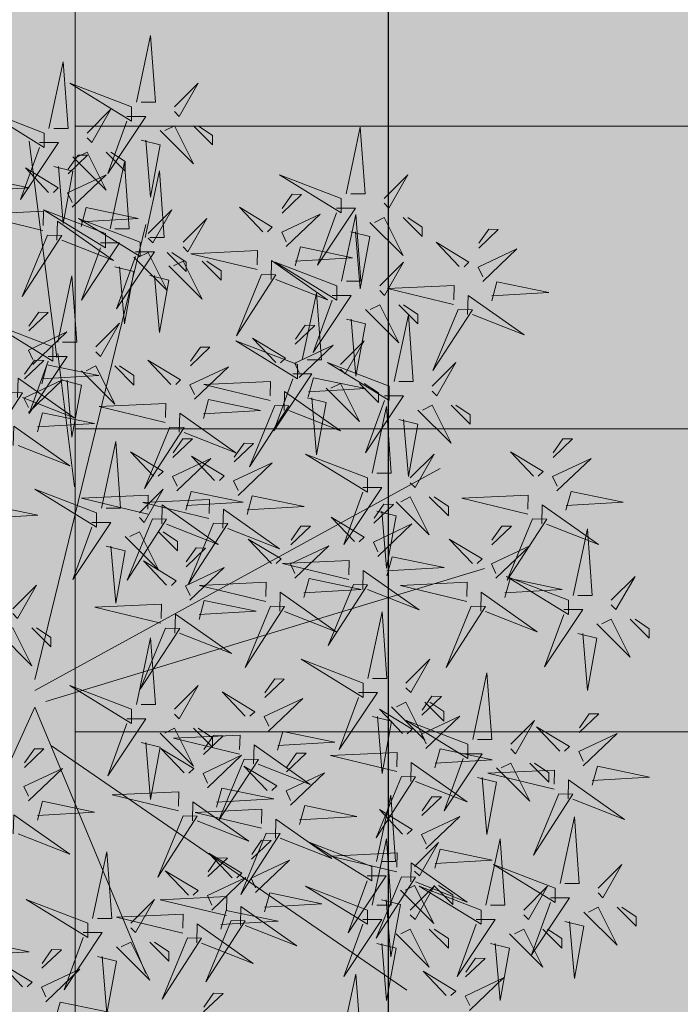
# Model space of a CAD drawing. Units: inches. Extents: x 1704 to 6393, y -157 to 1172.
# Tile 82 of 122: x 2064 to 2081, y 1006 to 1030. Entities that reach past the tile are written whole.
import ezdxf

# ---------------------------------------------------------------- set-up
doc = ezdxf.new("R2010")
doc.units = ezdxf.units.IN
doc.header["$MEASUREMENT"] = 0
for name, color, linetype, lineweight in [('A-ANNO-DIMS', 7, 'Continuous', 13), ('L-DECK-PLNK-PATT', 250, 'Continuous', 13), ('L-HRDS', 8, 'Continuous', 18), ('L-shrub', 74, 'Continuous', 18)]:
    doc.layers.add(name, color=color, linetype=linetype, lineweight=lineweight)
doc.layers.add('L-DECK-PATT', color=35, linetype='Continuous', lineweight=13, true_color=0xa6725b)
doc.layers.add('L-HRDS-PATT', color=9, linetype='Continuous', lineweight=13, true_color=0xc5c1ba)
doc.styles.get("Standard").update_dxf_attribs({"font": 'arial.ttf'})
doc.dimstyles.get("Standard").update_dxf_attribs({"dimtxt": 6, "dimasz": 2, "dimexe": 0.18, "dimexo": 0.0625, "dimgap": 0.09, "dimtad": 0, "dimtih": 1, "dimtoh": 1, "dimdec": 1, "dimzin": 0, "dimdsep": 46, "dimlunit": 3, "dimtxsty": 'Standard', "dimblk": 'ARCHTICK', "dimcen": 0.09, "dimadec": 0, "dimazin": 0, "dimtfac": 1, "dimtdec": 1, "dimtofl": 0, "dimtmove": 0, "dimatfit": 3, "dimfxl": 1, "dimtolj": 1, "dimtzin": 0, "dimarcsym": 0})

# ---------------------------------------------------------------- blocks, each defined once
blk = doc.blocks.new('shrub3')
for p, q in [((-5.99, -2.5), (58.67, 140.12)), ((-14.08, 16.34), (-186.51, 134.74)), ((-5.99, -2.5), (-59.88, 126.66)), ((-11.38, -5.19), (-224.23, -69.78)), ((-5.99, -10.57), (-202.68, -118.21)), ((-5.99, -15.96), (-59.88, -236.62)), ((-17.27, -174.02), (-25.36, -109.43)), ((-16.77, -172.03), (-3.3, -276.98))]:
    blk.add_line(p, q)
for points in [[(-154.93, 159.27), (-161.86, 126.99), (-164.17, 159.27), (-157.24, 159.27)], [(-15.75, 149.73), (-18.28, 140.55), (-43.52, 145.8), (-15.81, 147.42)], [(-217.01, 144.61), (-233.55, 128.86), (-214.88, 137.63), (-217.07, 142.31)], [(-87.91, 145.34), (-97.36, 136.34), (-92.75, 136.22), (-87.97, 143.03)], [(-36.4, 118.43), (-45.64, 120.73), (-41.02, 146.1), (-38.71, 118.43)], [(-227.2, 112.08), (-236.44, 114.38), (-231.82, 139.75), (-229.51, 112.08)], [(-172.08, 112.08), (-181.32, 114.38), (-176.7, 139.75), (-174.39, 112.08)], [(-80.06, 109.47), (-67.78, 139.19), (-86.97, 109.65), (-80.06, 109.47)], [(-11.37, 140.38), (-27.91, 124.63), (-9.24, 133.4), (-11.43, 138.07)], [(-205.66, 137.4), (-194.42, 125.57), (-210.33, 135.21), (-207.96, 137.46)], [(-29.48, 106.9), (-38.71, 106.9), (-20.24, 134.57), (-29.48, 109.2)], [(-263.24, 101.49), (-272.48, 103.79), (-267.86, 129.16), (-265.55, 101.49)], [(-101.26, 101), (-88.98, 130.72), (-108.17, 101.18), (-101.26, 101)], [(-45.64, 113.82), (-61.8, 129.96), (-52.56, 111.51), (-47.94, 113.82)], [(-0.02, 133.17), (11.22, 121.34), (-4.68, 130.97), (-2.32, 133.22)], [(-220.28, 100.55), (-229.51, 100.55), (-211.04, 128.22), (-220.28, 102.85)], [(-215.11, 128.4), (-224.56, 119.4), (-219.95, 119.28), (-215.17, 126.09)], [(-165.16, 100.55), (-174.39, 100.55), (-155.92, 128.22), (-165.16, 102.85)], [(-236.44, 107.46), (-252.6, 123.6), (-243.36, 105.16), (-238.75, 107.46)], [(-181.32, 107.46), (-197.48, 123.6), (-188.24, 105.16), (-183.63, 107.46)], [(-84.61, 111.9), (-84.84, 102.66), (-112.04, 121.82), (-86.91, 111.95)], [(-61.8, 111.51), (-71.03, 120.73), (-71.03, 116.12), (-64.1, 111.51)], [(-9.47, 124.17), (-18.92, 115.16), (-14.31, 115.05), (-9.53, 121.86)], [(24.53, 120.08), (22, 110.91), (-3.24, 116.16), (24.47, 117.77)], [(-256.32, 89.96), (-265.55, 89.96), (-247.08, 117.63), (-256.32, 92.27)], [(-174.2, 90.9), (-183.44, 93.21), (-178.82, 118.57), (-176.51, 90.9)], [(-272.48, 96.88), (-288.64, 113.02), (-279.4, 94.57), (-274.79, 96.88)], [(-252.6, 105.16), (-261.83, 114.38), (-261.83, 109.77), (-254.91, 105.16)], [(-197.48, 105.16), (-206.71, 114.38), (-206.71, 109.77), (-199.79, 105.16)], [(-105.81, 103.43), (-106.04, 94.19), (-133.24, 113.35), (-108.11, 103.48)], [(-183.94, 79.83), (-171.66, 109.54), (-190.85, 80), (-183.94, 79.83)], [(-167.28, 79.37), (-176.51, 79.37), (-158.04, 107.04), (-167.28, 81.68)], [(-96.31, 105.26), (-98.84, 96.09), (-124.08, 101.34), (-96.37, 102.95)], [(-77.81, 107.11), (-45.71, 99.37), (-78.04, 97.87), (-77.87, 104.8)], [(-52.56, 102.29), (-64.1, 90.76), (-54.87, 106.9), (-52.56, 104.59)], [(-31.78, 102.29), (-1.77, 90.76), (-31.78, 109.2), (-31.78, 102.29)], [(-288.64, 94.57), (-297.87, 103.79), (-297.87, 99.18), (-290.95, 94.57)], [(-243.36, 95.94), (-254.91, 84.41), (-245.67, 100.55), (-243.36, 98.24)], [(-222.59, 95.94), (-192.57, 84.41), (-222.59, 102.85), (-222.59, 95.94)], [(-188.24, 95.94), (-199.79, 84.41), (-190.55, 100.55), (-188.24, 98.24)], [(-183.44, 86.29), (-199.6, 102.43), (-190.36, 83.98), (-185.75, 86.29)], [(-167.46, 95.94), (-137.45, 84.41), (-167.46, 102.85), (-167.46, 95.94)], [(-117.51, 96.79), (-120.04, 87.62), (-145.28, 92.87), (-117.57, 94.48)], [(-91.93, 95.91), (-108.47, 80.16), (-89.8, 88.93), (-91.99, 93.61)], [(-99.01, 98.64), (-66.91, 90.91), (-99.24, 89.41), (-99.07, 96.33)], [(-34.09, 99.98), (-41.02, 67.7), (-43.33, 99.98), (-36.4, 99.98)], [(-258.63, 85.35), (-228.61, 73.82), (-258.63, 92.27), (-258.63, 85.35)], [(-224.89, 93.63), (-231.82, 61.35), (-234.13, 93.63), (-227.2, 93.63)], [(-188.49, 82.25), (-188.72, 73.02), (-215.92, 92.18), (-190.8, 82.31)], [(-199.6, 83.98), (-208.83, 93.21), (-208.83, 88.6), (-201.91, 83.98)], [(-169.77, 93.63), (-176.7, 61.35), (-179.01, 93.63), (-172.08, 93.63)], [(-279.4, 85.35), (-290.95, 73.82), (-281.71, 89.96), (-279.4, 87.65)], [(-113.13, 87.44), (-129.67, 71.69), (-111, 80.46), (-113.19, 85.14)], [(-118.22, 58.65), (-105.94, 88.37), (-125.13, 58.83), (-118.22, 58.65)], [(-80.58, 88.7), (-69.34, 76.87), (-85.25, 86.51), (-82.88, 88.76)], [(-260.93, 83.04), (-267.86, 50.76), (-270.17, 83.04), (-263.24, 83.04)], [(-169.58, 74.76), (-139.57, 63.23), (-169.58, 81.68), (-169.58, 74.76)], [(-190.36, 74.76), (-201.91, 63.23), (-192.67, 79.37), (-190.36, 77.07)], [(-181.69, 77.46), (-149.59, 69.73), (-181.92, 68.23), (-181.75, 75.15)], [(-101.78, 80.23), (-90.54, 68.4), (-106.45, 78.04), (-104.08, 80.29)], [(-90.03, 79.7), (-99.48, 70.7), (-94.87, 70.58), (-90.09, 77.39)], [(-77.94, 50.18), (-65.66, 79.9), (-84.85, 50.36), (-77.94, 50.18)], [(-200.19, 75.62), (-202.73, 66.44), (-227.97, 71.69), (-200.25, 73.31)], [(-171.89, 72.46), (-178.82, 40.17), (-181.13, 72.46), (-174.2, 72.46)], [(-260.26, 39.6), (-247.98, 69.31), (-267.17, 39.77), (-260.26, 39.6)], [(-122.77, 61.08), (-123, 51.85), (-150.2, 71), (-125.08, 61.14)], [(-111.23, 71.23), (-120.68, 62.23), (-116.07, 62.11), (-111.29, 68.92)], [(4.43, 58.96), (4.2, 49.73), (-23, 68.88), (2.13, 59.02)], [(-195.81, 66.27), (-212.35, 50.52), (-193.68, 59.29), (-195.87, 63.96)], [(-82.49, 52.61), (-82.72, 43.38), (-109.92, 62.53), (-84.79, 52.67)], [(-220.84, 31.61), (-230.08, 33.92), (-225.46, 59.28), (-223.15, 31.61)], [(-183.94, 31.13), (-171.66, 60.84), (-190.85, 31.3), (-183.94, 31.13)], [(-184.46, 59.06), (-173.22, 47.23), (-189.13, 56.86), (-186.76, 59.12)], [(-134.47, 54.44), (-137, 45.27), (-162.24, 50.52), (-134.53, 52.13)], [(-115.97, 56.29), (-83.87, 48.56), (-116.2, 47.06), (-116.03, 53.98)], [(-264.81, 42.02), (-265.04, 32.79), (-292.24, 51.95), (-267.12, 42.08)], [(-193.91, 50.06), (-203.36, 41.06), (-198.75, 40.94), (-193.97, 47.75)], [(-107.62, 22.66), (-95.34, 52.37), (-114.53, 22.83), (-107.62, 22.66)], [(-75.69, 47.82), (-43.59, 40.09), (-75.92, 38.59), (-75.75, 45.51)], [(-7.27, 52.33), (-9.8, 43.15), (-35.04, 48.4), (-7.33, 50.02)], [(-230.08, 27), (-246.24, 43.14), (-237, 24.7), (-232.39, 27)], [(-213.92, 20.09), (-223.15, 20.09), (-204.68, 47.76), (-213.92, 22.39)], [(-188.49, 33.55), (-188.72, 24.32), (-215.92, 43.48), (-190.8, 33.61)], [(-130.09, 45.1), (-146.63, 29.34), (-127.96, 38.11), (-130.15, 42.79)], [(-94.19, 45.97), (-96.72, 36.8), (-121.96, 42.05), (-94.25, 43.67)], [(-57.6, 14.68), (-66.84, 16.98), (-62.22, 42.34), (-59.91, 14.68)], [(-2.89, 42.98), (-19.43, 27.23), (-0.76, 36), (-2.95, 40.67)], [(-276.51, 35.39), (-279.05, 26.21), (-304.29, 31.46), (-276.57, 33.08)], [(-258.01, 37.23), (-225.91, 29.5), (-258.24, 28), (-258.07, 34.92)], [(-246.24, 24.7), (-255.47, 33.92), (-255.47, 29.31), (-248.55, 24.7)], [(-112.17, 25.08), (-112.4, 15.85), (-139.6, 35.01), (-114.47, 25.14)], [(-118.74, 37.88), (-107.5, 26.06), (-123.41, 35.69), (-121.04, 37.94)], [(-89.81, 36.63), (-106.35, 20.87), (-87.68, 29.64), (-89.87, 34.32)], [(-181.69, 28.76), (-149.59, 21.03), (-181.92, 19.53), (-181.75, 26.45)], [(-169.96, 1.97), (-179.2, 4.28), (-174.58, 29.64), (-172.27, 1.97)], [(-128.19, 28.88), (-137.64, 19.88), (-133.03, 19.77), (-128.25, 26.57)], [(-78.46, 29.41), (-67.22, 17.59), (-83.13, 27.22), (-80.76, 29.47)], [(-50.68, 3.15), (-59.91, 3.15), (-41.44, 30.82), (-50.68, 5.45)], [(-272.13, 26.04), (-288.67, 10.29), (-270, 19.06), (-272.19, 23.73)], [(-200.19, 26.92), (-202.73, 17.74), (-227.97, 22.99), (-200.25, 24.61)], [(-66.84, 10.06), (-83, 26.2), (-73.76, 7.76), (-69.14, 10.06)], [(-0.99, 26.77), (-10.44, 17.76), (-5.83, 17.65), (-1.05, 24.46)], [(-237, 15.47), (-248.55, 3.95), (-239.31, 20.09), (-237, 17.78)], [(-216.23, 15.47), (-186.21, 3.95), (-216.23, 22.39), (-216.23, 15.47)], [(-105.37, 20.29), (-73.27, 12.56), (-105.6, 11.06), (-105.43, 17.99)], [(-87.91, 20.41), (-97.36, 11.41), (-92.75, 11.3), (-87.97, 18.11)], [(-260.78, 18.83), (-249.54, 7), (-265.45, 16.63), (-263.08, 18.88)], [(-195.81, 17.57), (-212.35, 1.82), (-193.68, 10.59), (-195.87, 15.26)], [(-163.04, -9.56), (-172.27, -9.56), (-153.8, 18.11), (-163.04, -7.25)], [(-123.87, 18.45), (-126.4, 9.27), (-151.64, 14.52), (-123.93, 16.14)], [(-83, 7.76), (-92.23, 16.98), (-92.23, 12.37), (-85.3, 7.76)], [(-270.23, 9.83), (-279.68, 0.83), (-275.07, 0.71), (-270.29, 7.52)], [(-218.53, 13.17), (-225.46, -19.11), (-227.77, 13.17), (-220.84, 13.17)], [(-179.2, -2.64), (-195.36, 13.5), (-186.12, -4.95), (-181.51, -2.64)], [(-184.46, 10.36), (-173.22, -1.47), (-189.13, 8.16), (-186.76, 10.41)], [(-119.49, 9.1), (-136.03, -6.65), (-117.36, 2.12), (-119.55, 6.79)], [(-52.98, -1.46), (-22.97, -12.99), (-52.98, 5.45), (-52.98, -1.46)], [(-195.36, -4.95), (-204.59, 4.28), (-204.59, -0.33), (-197.67, -4.95)], [(-193.91, 1.36), (-203.36, -7.64), (-198.75, -7.76), (-193.97, -0.95)], [(-108.14, 1.89), (-96.9, -9.94), (-112.81, -0.3), (-110.44, 1.95)], [(-73.76, -1.46), (-85.3, -12.99), (-76.07, 3.15), (-73.76, 0.84)], [(-55.29, -3.77), (-62.22, -36.05), (-64.53, -3.77), (-57.6, -3.77)], [(-165.34, -14.17), (-135.33, -25.7), (-165.34, -7.25), (-165.34, -14.17)], [(-117.59, -7.11), (-127.04, -16.11), (-122.43, -16.23), (-117.65, -9.42)], [(-269.6, -38.26), (-278.84, -35.95), (-274.22, -10.59), (-271.91, -38.26)], [(-186.12, -14.17), (-197.67, -25.7), (-188.43, -9.56), (-186.12, -11.86)], [(-69.46, -40.86), (-57.18, -11.15), (-76.37, -40.69), (-69.46, -40.86)], [(-167.65, -16.47), (-174.58, -48.76), (-176.89, -16.47), (-169.96, -16.47)], [(-262.68, -49.79), (-271.91, -49.79), (-253.44, -22.12), (-262.68, -47.48)], [(-217.86, -51.45), (-205.58, -21.74), (-224.77, -51.28), (-217.86, -51.45)], [(-120.34, -51.45), (-108.06, -21.74), (-127.25, -51.28), (-120.34, -51.45)], [(11.6, -38.64), (-4.56, -22.5), (4.68, -40.94), (9.3, -38.64)], [(-278.84, -42.87), (-295, -26.73), (-285.76, -45.18), (-281.15, -42.87)], [(-74.01, -38.44), (-74.24, -47.67), (-101.44, -28.52), (-76.31, -38.38)], [(-160.62, -62.04), (-148.34, -32.32), (-167.53, -61.86), (-160.62, -62.04)], [(-4.56, -40.94), (-13.79, -31.72), (-13.79, -36.33), (-6.86, -40.94)], [(-295, -45.18), (-304.23, -35.95), (-304.23, -40.56), (-297.31, -45.18)], [(-222.41, -49.03), (-222.64, -58.26), (-249.84, -39.1), (-224.72, -48.97)], [(-124.89, -49.03), (-125.12, -58.26), (-152.32, -39.1), (-127.2, -48.97)], [(-264.99, -54.4), (-234.97, -65.93), (-264.99, -47.48), (-264.99, -54.4)], [(-85.71, -45.07), (-88.24, -54.25), (-113.48, -49), (-85.77, -47.38)], [(-67.21, -43.23), (-35.11, -50.96), (-67.44, -52.46), (-67.27, -45.54)], [(4.68, -50.16), (-6.86, -61.69), (2.37, -45.55), (4.68, -47.86)], [(-285.76, -54.4), (-297.31, -65.93), (-288.07, -49.79), (-285.76, -52.09)], [(-165.17, -59.61), (-165.4, -68.85), (-192.6, -49.69), (-167.48, -59.56)], [(-267.29, -56.71), (-274.22, -88.99), (-276.53, -56.71), (-269.6, -56.71)], [(-234.11, -55.66), (-236.65, -64.84), (-261.89, -59.59), (-234.17, -57.97)], [(-215.61, -53.82), (-183.51, -61.55), (-215.84, -63.05), (-215.67, -56.12)], [(-136.59, -55.66), (-139.12, -64.84), (-164.36, -59.59), (-136.65, -57.97)], [(-118.09, -53.82), (-85.99, -61.55), (-118.32, -63.05), (-118.15, -56.12)], [(-81.33, -54.42), (-97.87, -70.17), (-79.2, -61.4), (-81.39, -56.73)], [(-40.64, -80.61), (-49.88, -78.3), (-45.26, -52.94), (-42.95, -80.61)], [(-92.78, -91.68), (-80.5, -61.97), (-99.69, -91.51), (-92.78, -91.68)], [(-69.98, -61.63), (-58.74, -73.46), (-74.65, -63.83), (-72.28, -61.58)], [(-247.54, -93.8), (-235.26, -64.08), (-254.45, -93.62), (-247.54, -93.8)], [(-229.73, -65.01), (-246.27, -80.76), (-227.6, -71.99), (-229.79, -67.32)], [(-176.87, -66.25), (-179.4, -75.42), (-204.64, -70.17), (-176.93, -68.56)], [(-158.37, -64.4), (-126.27, -72.13), (-158.6, -73.63), (-158.43, -66.71)], [(-132.21, -65.01), (-148.75, -80.76), (-130.08, -71.99), (-132.27, -67.32)], [(-63.1, -93.8), (-50.82, -64.08), (-70.01, -93.62), (-63.1, -93.8)], [(-33.72, -92.14), (-42.95, -92.14), (-24.48, -64.47), (-33.72, -89.83)], [(-172.08, -97.55), (-181.32, -95.24), (-176.7, -69.88), (-174.39, -97.55)], [(-79.43, -70.63), (-88.88, -79.64), (-84.27, -79.75), (-79.49, -72.94)], [(-49.88, -85.22), (-66.04, -69.08), (-56.8, -87.52), (-52.18, -85.22)], [(-218.38, -72.22), (-207.14, -84.05), (-223.05, -74.41), (-220.68, -72.16)], [(-172.49, -75.6), (-189.03, -91.35), (-170.36, -82.58), (-172.55, -77.9)], [(-120.86, -72.22), (-109.62, -84.05), (-125.53, -74.41), (-123.16, -72.16)], [(-97.33, -89.26), (-97.56, -98.49), (-124.76, -79.33), (-99.63, -89.2)], [(-66.04, -87.52), (-75.27, -78.3), (-75.27, -82.91), (-68.34, -87.52)], [(-252.09, -91.37), (-252.32, -100.61), (-279.52, -81.45), (-254.4, -91.32)], [(-227.83, -81.22), (-237.28, -90.22), (-232.67, -90.34), (-227.89, -83.53)], [(-165.16, -109.08), (-174.39, -109.08), (-155.92, -81.41), (-165.16, -106.77)], [(-161.14, -82.81), (-149.9, -94.64), (-165.81, -85), (-163.44, -82.75)], [(-130.31, -81.22), (-139.76, -90.22), (-135.15, -90.34), (-130.37, -83.53)], [(-67.65, -91.37), (-67.88, -100.61), (-95.08, -81.45), (-69.95, -91.32)], [(-181.32, -102.16), (-197.48, -86.02), (-188.24, -104.46), (-183.63, -102.16)], [(-36.02, -96.75), (-6.01, -108.28), (-36.02, -89.83), (-36.02, -96.75)], [(-197.48, -104.46), (-206.71, -95.24), (-206.71, -99.85), (-199.79, -104.46)], [(-170.59, -91.81), (-180.04, -100.81), (-175.43, -100.93), (-170.65, -94.12)], [(-90.53, -94.05), (-58.43, -101.78), (-90.76, -103.28), (-90.59, -96.35)], [(-56.8, -96.75), (-68.34, -108.28), (-59.11, -92.14), (-56.8, -94.44)], [(20.29, -91.66), (17.76, -100.83), (-7.48, -95.58), (20.23, -93.97)], [(-263.79, -98.01), (-266.33, -107.18), (-291.57, -101.93), (-263.85, -100.32)], [(-245.29, -96.16), (-213.19, -103.89), (-245.52, -105.4), (-245.35, -98.47)], [(-109.03, -95.89), (-111.56, -105.07), (-136.8, -99.82), (-109.09, -98.2)], [(-79.35, -98.01), (-81.88, -107.18), (-107.12, -101.93), (-79.41, -100.32)], [(-60.85, -96.16), (-28.75, -103.89), (-61.08, -105.4), (-60.91, -98.47)], [(-38.33, -99.05), (-45.26, -131.33), (-47.57, -99.05), (-40.64, -99.05)], [(-259.41, -107.36), (-275.95, -123.11), (-257.28, -114.34), (-259.47, -109.66)], [(-188.24, -113.69), (-199.79, -125.22), (-190.55, -109.08), (-188.24, -111.38)], [(-167.46, -113.69), (-137.45, -125.22), (-167.46, -106.77), (-167.46, -113.69)], [(-104.65, -105.24), (-121.19, -120.99), (-102.52, -112.22), (-104.71, -107.55)], [(-74.97, -107.36), (-91.51, -123.11), (-72.84, -114.34), (-75.03, -109.66)], [(-71.58, -138.26), (-59.3, -108.55), (-78.49, -138.09), (-71.58, -138.26)], [(-248.06, -114.57), (-236.82, -126.4), (-252.73, -116.76), (-250.36, -114.51)], [(-182.68, -142.01), (-191.92, -139.71), (-187.3, -114.34), (-184.99, -142.01)], [(-93.3, -112.45), (-82.06, -124.28), (-97.97, -114.64), (-95.6, -112.39)], [(-63.62, -114.57), (-52.38, -126.4), (-68.29, -116.76), (-65.92, -114.51)], [(-169.77, -115.99), (-176.7, -148.27), (-179.01, -115.99), (-172.08, -115.99)], [(-122.46, -148.85), (-110.18, -119.14), (-129.37, -148.68), (-122.46, -148.85)], [(-257.51, -123.57), (-266.96, -132.57), (-262.35, -132.69), (-257.57, -125.88)], [(-102.75, -121.45), (-112.2, -130.45), (-107.59, -130.57), (-102.81, -123.76)], [(-73.07, -123.57), (-82.52, -132.57), (-77.91, -132.69), (-73.13, -125.88)], [(4.43, -129.49), (4.2, -138.72), (-23, -119.56), (2.13, -129.43)], [(-175.76, -153.54), (-184.99, -153.54), (-166.52, -125.87), (-175.76, -151.23)], [(-138.16, -152.6), (-147.4, -150.29), (-142.78, -124.93), (-140.47, -152.6)], [(-76.13, -135.84), (-76.36, -145.07), (-103.56, -125.92), (-78.43, -135.78)], [(6.86, -155.2), (19.14, -125.49), (-0.05, -155.03), (6.86, -155.2)], [(-191.92, -146.62), (-208.08, -130.48), (-198.84, -148.93), (-194.23, -146.62)], [(-19.44, -161.07), (-28.68, -158.76), (-24.06, -133.4), (-21.75, -161.07)], [(-127.01, -146.43), (-127.24, -155.66), (-154.44, -136.5), (-129.32, -146.37)], [(-131.24, -164.13), (-140.47, -164.13), (-122, -136.46), (-131.24, -161.82)], [(-7.27, -136.12), (-9.8, -145.3), (-35.04, -140.05), (-7.33, -138.43)], [(-208.08, -148.93), (-217.31, -139.71), (-217.31, -144.32), (-210.39, -148.93)], [(-147.4, -157.21), (-163.56, -141.07), (-154.32, -159.52), (-149.71, -157.21)], [(-87.83, -142.48), (-90.36, -151.65), (-115.6, -146.4), (-87.89, -144.78)], [(-69.33, -140.63), (-37.23, -148.36), (-69.56, -149.86), (-69.39, -142.94)], [(2.31, -152.78), (2.08, -162.01), (-25.12, -142.86), (0.01, -152.72)], [(-12.52, -172.6), (-21.75, -172.6), (-3.28, -144.93), (-12.52, -170.29)], [(-2.89, -145.47), (-19.43, -161.22), (-0.76, -152.45), (-2.95, -147.78)], [(-178.06, -158.15), (-148.05, -169.68), (-178.06, -151.23), (-178.06, -158.15)], [(-163.56, -159.52), (-172.79, -150.29), (-172.79, -154.9), (-165.87, -159.52)], [(-120.21, -151.22), (-88.11, -158.95), (-120.44, -160.45), (-120.27, -153.52)], [(-83.45, -151.82), (-99.99, -167.57), (-81.32, -158.8), (-83.51, -154.13)], [(-28.68, -165.68), (-44.84, -149.54), (-35.6, -167.99), (-30.98, -165.68)], [(-198.84, -158.15), (-210.39, -169.68), (-201.15, -153.54), (-198.84, -155.85)], [(-138.71, -153.06), (-141.24, -162.24), (-166.48, -156.99), (-138.77, -155.37)], [(-180.37, -160.46), (-187.3, -192.74), (-189.61, -160.46), (-182.68, -160.46)], [(-133.54, -168.74), (-103.53, -180.27), (-133.54, -161.82), (-133.54, -168.74)], [(-72.1, -159.03), (-60.86, -170.86), (-76.77, -161.23), (-74.4, -158.98)], [(-44.84, -167.99), (-54.07, -158.76), (-54.07, -163.37), (-47.14, -167.99)], [(-9.39, -159.41), (-11.92, -168.59), (-37.16, -163.34), (-9.45, -161.72)], [(-0.99, -161.68), (-10.44, -170.68), (-5.83, -170.8), (-1.05, -163.99)], [(-211.5, -195.43), (-199.22, -165.72), (-218.41, -195.26), (-211.5, -195.43)], [(-157.24, -190.71), (-166.48, -188.41), (-161.86, -163.04), (-159.55, -190.71)], [(-154.32, -168.74), (-165.87, -180.27), (-156.63, -164.13), (-154.32, -166.43)], [(-134.33, -162.41), (-150.87, -178.16), (-132.2, -169.39), (-134.39, -164.72)], [(-135.85, -171.04), (-142.78, -203.33), (-145.09, -171.04), (-138.16, -171.04)], [(-122.98, -169.62), (-111.74, -181.45), (-127.65, -171.81), (-125.28, -169.56)], [(-81.55, -168.04), (-91, -177.04), (-86.39, -177.15), (-81.61, -170.34)], [(-5.01, -168.76), (-21.55, -184.51), (-2.88, -175.74), (-5.07, -171.07)], [(-14.82, -177.21), (15.19, -188.74), (-14.82, -170.29), (-14.82, -177.21)], [(-150.32, -202.24), (-159.55, -202.24), (-141.08, -174.57), (-150.32, -199.93)], [(-35.6, -177.21), (-47.14, -188.74), (-37.91, -172.6), (-35.6, -174.9)], [(-166.48, -195.32), (-182.64, -179.18), (-173.4, -197.63), (-168.79, -195.32)], [(-132.43, -178.62), (-141.88, -187.62), (-137.27, -187.74), (-132.49, -180.93)], [(-17.13, -179.51), (-24.06, -211.79), (-26.37, -179.51), (-19.44, -179.51)], [(-216.05, -193.01), (-216.28, -202.24), (-243.48, -183.09), (-218.36, -192.95)], [(-116.1, -212.37), (-103.82, -182.66), (-123.01, -212.2), (-116.1, -212.37)], [(-61.84, -211.89), (-71.08, -209.58), (-66.46, -184.22), (-64.15, -211.89)], [(-3.11, -184.97), (-12.56, -193.97), (-7.95, -194.09), (-3.17, -187.28)], [(-182.64, -197.63), (-191.87, -188.41), (-191.87, -193.02), (-184.95, -197.63)], [(-44.88, -216.12), (-54.12, -213.81), (-49.5, -188.45), (-47.19, -216.12)], [(-54.92, -223.41), (-64.15, -223.41), (-45.68, -195.75), (-54.92, -221.11)], [(-227.75, -199.64), (-230.29, -208.82), (-255.53, -203.57), (-227.81, -201.95)], [(-209.25, -197.8), (-177.15, -205.53), (-209.48, -207.03), (-209.31, -200.11)], [(-152.62, -206.85), (-122.61, -218.38), (-152.62, -199.93), (-152.62, -206.85)], [(-120.65, -209.95), (-120.88, -219.18), (-148.08, -200.02), (-122.96, -209.89)], [(-71.08, -216.5), (-87.24, -200.36), (-78, -218.8), (-73.38, -216.5)], [(-37.96, -227.65), (-47.19, -227.65), (-28.72, -199.98), (-37.96, -225.34)], [(-173.4, -206.85), (-184.95, -218.38), (-175.71, -202.24), (-173.4, -204.55)], [(-54.12, -220.73), (-70.28, -204.59), (-61.04, -223.04), (-56.42, -220.73)], [(-12.22, -231.43), (0.06, -201.71), (-19.13, -231.26), (-12.22, -231.43)], [(-223.37, -208.99), (-239.91, -224.74), (-221.24, -215.97), (-223.43, -211.3)], [(-159.36, -233.06), (-168.6, -230.75), (-163.98, -205.39), (-161.67, -233.06)], [(-154.93, -209.16), (-161.86, -241.44), (-164.17, -209.16), (-157.24, -209.16)], [(-87.24, -218.8), (-96.47, -209.58), (-96.47, -214.19), (-89.54, -218.8)], [(-113.85, -214.74), (-81.75, -222.47), (-114.08, -223.97), (-113.91, -217.05)], [(-70.28, -223.04), (-79.51, -213.81), (-79.51, -218.43), (-72.58, -223.04)], [(-212.02, -216.2), (-200.78, -228.03), (-216.69, -218.4), (-214.32, -216.15)], [(-152.44, -244.59), (-161.67, -244.59), (-143.2, -216.92), (-152.44, -242.28)], [(-132.35, -216.58), (-134.88, -225.76), (-160.12, -220.51), (-132.41, -218.89)], [(-16.77, -229.01), (-17, -238.24), (-44.2, -219.08), (-19.07, -228.95)], [(-168.6, -237.67), (-184.76, -221.53), (-175.52, -239.98), (-170.91, -237.67)], [(-78, -228.03), (-89.54, -239.55), (-80.31, -223.41), (-78, -225.72)], [(-57.22, -228.03), (-27.21, -239.55), (-57.22, -221.11), (-57.22, -228.03)], [(-221.47, -225.2), (-230.92, -234.21), (-226.31, -234.32), (-221.53, -227.51)], [(-127.97, -225.93), (-144.51, -241.68), (-125.84, -232.91), (-128.03, -228.24)], [(-61.04, -232.26), (-72.58, -243.79), (-63.35, -227.65), (-61.04, -229.95)], [(-40.26, -232.26), (-10.25, -243.79), (-40.26, -225.34), (-40.26, -232.26)], [(-184.76, -239.98), (-193.99, -230.75), (-193.99, -235.37), (-187.07, -239.98)], [(-116.62, -233.14), (-105.38, -244.97), (-121.29, -235.34), (-118.92, -233.09)], [(-59.53, -230.33), (-66.46, -262.61), (-68.77, -230.33), (-61.84, -230.33)], [(-9.97, -233.79), (22.13, -241.53), (-10.2, -243.03), (-10.03, -236.1)], [(-28.47, -235.64), (-31, -244.81), (-56.24, -239.56), (-28.53, -237.95)], [(-42.57, -234.57), (-49.5, -266.85), (-51.81, -234.57), (-44.88, -234.57)], [(-15.2, -264.82), (-24.44, -262.51), (-19.82, -237.15), (-17.51, -264.82)], [(-154.74, -249.2), (-124.73, -260.73), (-154.74, -242.28), (-154.74, -249.2)], [(-126.07, -242.14), (-135.52, -251.14), (-130.91, -251.26), (-126.13, -244.45)], [(-175.52, -249.2), (-187.07, -260.73), (-177.83, -244.59), (-175.52, -246.89)], [(-24.09, -244.99), (-40.63, -260.74), (-21.96, -251.97), (-24.15, -247.3)], [(-157.05, -251.51), (-163.98, -283.79), (-166.29, -251.51), (-159.36, -251.51)], [(-57.6, -277.52), (-66.84, -275.22), (-62.22, -249.86), (-59.91, -277.52)], [(-8.28, -276.35), (-17.51, -276.35), (0.96, -248.68), (-8.28, -274.04)], [(-12.74, -252.2), (-1.5, -264.03), (-17.4, -254.39), (-15.04, -252.14)], [(24.53, -250.46), (22, -259.64), (-3.24, -254.39), (24.47, -252.77)], [(-24.44, -269.43), (-40.6, -253.29), (-31.36, -271.74), (-26.74, -269.43)], [(-50.68, -289.05), (-59.91, -289.05), (-41.44, -261.38), (-50.68, -286.75)], [(-40.6, -271.74), (-49.83, -262.51), (-49.83, -267.13), (-42.9, -271.74)], [(-22.19, -261.2), (-31.64, -270.2), (-27.03, -270.32), (-22.25, -263.51)], [(-66.84, -282.14), (-83, -266), (-73.76, -284.44), (-69.14, -282.14)], [(-83, -284.44), (-92.23, -275.22), (-92.23, -279.83), (-85.3, -284.44)], [(-31.36, -280.96), (-42.9, -292.49), (-33.67, -276.35), (-31.36, -278.65)], [(-10.58, -280.96), (19.43, -292.49), (-10.58, -274.04), (-10.58, -280.96)], [(-12.89, -283.27), (-19.82, -315.55), (-22.13, -283.27), (-15.2, -283.27)], [(-73.76, -293.67), (-85.3, -305.19), (-76.07, -289.05), (-73.76, -291.36)], [(-52.98, -293.67), (-22.97, -305.19), (-52.98, -286.75), (-52.98, -293.67)], [(-55.29, -295.97), (-62.22, -328.25), (-64.53, -295.97), (-57.6, -295.97)]]:
    blk.add_lwpolyline(points)
blk = doc.blocks.new('_ArchTick')
at = {"color": 0, "linetype": 'ByBlock', "const_width": 0.15}
blk.add_lwpolyline([(-0.5, -0.5), (0.5, 0.5)], dxfattribs=at)
blk = doc.blocks.new('*D92')
at = {"layer": 'A-ANNO-DIMS', "color": 0, "lineweight": -2, "transparency": 16777216}
for p, q in [((2073.349, 895.275), (2073.349, 1105.287)), ((2605.349, 895.275), (2605.349, 1105.287)), ((2073.349, 1105.107), (2332.661, 1105.107)), ((2605.349, 1105.107), (2346.036, 1105.107))]:
    blk.add_line(p, q, dxfattribs=at)
at = {"layer": 'Defpoints', "color": 0, "lineweight": -3, "transparency": 16777216}
for p in [(2605.349, 1105.107), (2073.349, 895.213), (2605.349, 895.213)]:
    blk.add_point(p, dxfattribs=at)
at = {"layer": 'A-ANNO-DIMS', "color": 0, "lineweight": -2, "transparency": 16777216, "xscale": 2, "yscale": 2, "zscale": 2, "rotation": 180}
blk.add_blockref('_ArchTick', (2073.349, 1105.107), dxfattribs=at)
at = {"layer": 'A-ANNO-DIMS', "color": 0, "lineweight": -2, "transparency": 16777216, "xscale": 2, "yscale": 2, "zscale": 2}
blk.add_blockref('_ArchTick', (2605.349, 1105.107), dxfattribs=at)
at = {"layer": 'A-ANNO-DIMS', "color": 0, "transparency": 16777216, "insert": (2339.349, 1105.107), "char_height": 6, "attachment_point": 5}
blk.add_mtext('\\A1;532', dxfattribs=at)
blk = doc.blocks.new('*D94')
at = {"layer": 'A-ANNO-DIMS', "color": 0, "lineweight": -2, "transparency": 16777216}
for p, q in [((1898.349, 895.275), (1898.349, 1105.287)), ((2073.349, 895.275), (2073.349, 1105.287)), ((1898.349, 1105.107), (1979.39, 1105.107)), ((2073.349, 1105.107), (1992.307, 1105.107))]:
    blk.add_line(p, q, dxfattribs=at)
at = {"layer": 'Defpoints', "color": 0, "lineweight": -3, "transparency": 16777216}
for p in [(2073.349, 1105.107), (1898.349, 895.213), (2073.349, 895.213)]:
    blk.add_point(p, dxfattribs=at)
at = {"layer": 'A-ANNO-DIMS', "color": 0, "lineweight": -2, "transparency": 16777216, "xscale": 2, "yscale": 2, "zscale": 2, "rotation": 180}
blk.add_blockref('_ArchTick', (1898.349, 1105.107), dxfattribs=at)
at = {"layer": 'A-ANNO-DIMS', "color": 0, "lineweight": -2, "transparency": 16777216, "xscale": 2, "yscale": 2, "zscale": 2}
blk.add_blockref('_ArchTick', (2073.349, 1105.107), dxfattribs=at)
at = {"layer": 'A-ANNO-DIMS', "color": 0, "transparency": 16777216, "insert": (1985.849, 1105.107), "char_height": 6, "attachment_point": 5}
blk.add_mtext('\\A1;175', dxfattribs=at)

msp = doc.modelspace()

# ---------------------------------------------------------------- hatches: boundary and pattern name
at = {"layer": 'L-DECK-PATT', "transparency": 33554544}
h = msp.add_hatch(color=256, dxfattribs=at)
h.dxf.hatch_style = 1
h.paths.add_polyline_path([(2329.589, 1033.213), (2065.589, 1033.213), (2065.589, 895.213), (2167.349, 895.213), (2263.349, 895.213), (2263.349, 903.213), (2273.349, 903.213), (2273.349, 895.213), (2329.589, 895.213)])
h.paths.add_polyline_path([(2664.349, 1033.213), (2333.589, 1033.213), (2333.589, 895.213), (2465.349, 895.213), (2469.181, 895.213), (2470.482, 895.213), (2508.215, 895.213), (2509.516, 895.213), (2513.349, 895.213), (2533.349, 895.213), (2581.349, 895.213), (2605.349, 895.213), (2664.349, 895.213)])
h.paths.add_polyline_path([(2333.589, 1033.213), (2329.589, 1033.213), (2329.589, 895.213), (2333.589, 895.213)])
at = {"layer": 'L-DECK-PLNK-PATT'}
h = msp.add_hatch(dxfattribs=at)
h.set_pattern_fill('LINE', color=256, scale=60)
h.paths.add_polyline_path([(2329.589, 1033.213), (2065.589, 1033.213), (2065.589, 895.213), (2167.349, 895.213), (2263.349, 895.213), (2263.349, 903.213), (2273.349, 903.213), (2273.349, 895.213), (2329.589, 895.213)])
h.paths.add_polyline_path([(2664.349, 1033.213), (2333.589, 1033.213), (2333.589, 895.213), (2465.349, 895.213), (2469.181, 895.213), (2470.482, 895.213), (2508.215, 895.213), (2509.516, 895.213), (2513.349, 895.213), (2533.349, 895.213), (2581.349, 895.213), (2605.349, 895.213), (2664.349, 895.213)])
h.paths.add_polyline_path([(2333.589, 1033.213), (2329.589, 1033.213), (2329.589, 895.213), (2333.589, 895.213)])
at = {"layer": 'L-HRDS-PATT', "transparency": 33554643}
h = msp.add_hatch(color=256, dxfattribs=at)
h.dxf.hatch_style = 1
h.paths.add_polyline_path([(2065.589, 1033.213), (1898.349, 1033.213), (1898.349, 895.213), (2065.589, 895.213)])

# ---------------------------------------------------------------- linework, layer by layer
at = {"layer": 'L-HRDS'}
msp.add_line((2065.589, 895.213), (2065.589, 1033.213), dxfattribs=at)

# ---------------------------------------------------------------- block references
at = {"layer": 'L-shrub', "xscale": 0.0510581485411622, "yscale": 0.0510581485411622, "zscale": 0.0510581485411622, "rotation": 180}
msp.add_blockref('shrub3', (2064.28, 1012.986), dxfattribs=at)

# ---------------------------------------------------------------- dimensions: what is measured, and where the dimension line sits
at = {"layer": 'A-ANNO-DIMS'}
for base, p1, p2, picture, middle in [((2073.349, 1105.107), (1898.349, 895.213), (2073.349, 895.213), '*D94', (1985.849, 1105.107)), ((2605.349, 1105.107), (2073.349, 895.213), (2605.349, 895.213), '*D92', (2339.349, 1105.107))]:
    dim = msp.add_linear_dim(base=base, p1=p1, p2=p2, dimstyle='Standard', override={"dimdec": 0, "dimlfac": 1, "dimrnd": 0, "dimzin": 0, "dimdsep": 46, "dimlunit": 2}, dxfattribs=at)
    dim.commit()
    dim.dimension.update_dxf_attribs({"geometry": picture, "text_midpoint": middle})

doc.saveas('drawing.dxf')
